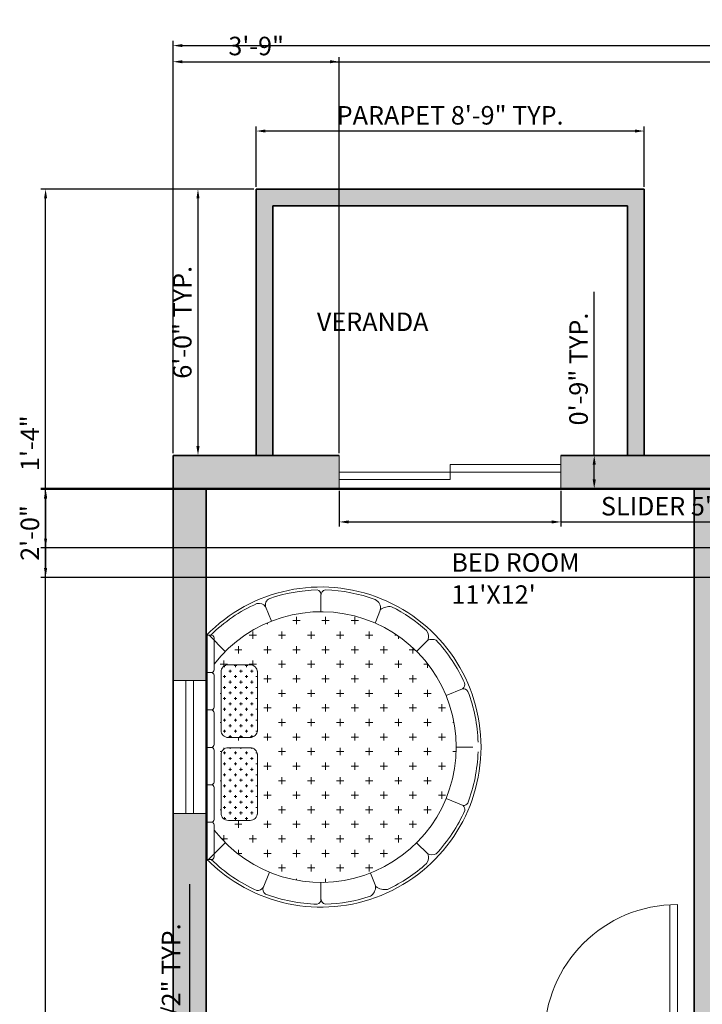
# Model space of a CAD drawing. Units: inches. Extents: x 2923 to 3500, y 1684 to 2381.
# Tile 10 of 12: x 2928 to 3112, y 2114 to 2380. Entities that reach past the tile are written whole.
import ezdxf

# ---------------------------------------------------------------- set-up
doc = ezdxf.new("R2010")
doc.units = ezdxf.units.IN
for name, color, linetype, lineweight in [('A-ANNO-DIMS', 2, 'Continuous', 18), ('A-AREA-IDEN', 7, 'Continuous', 18), ('A-DOOR', 3, 'Continuous', 18), ('A-FURN-PATT', 8, 'Continuous', 13), ('A-GLAZ', 4, 'Continuous', 18), ('A-WALL', 7, 'Continuous', 35), ('A-WALL-PATT', 9, 'Continuous', 13), ('Furniture', 7, 'Continuous', 15)]:
    doc.layers.add(name, color=color, linetype=linetype, lineweight=lineweight)
doc.styles.get("Standard").update_dxf_attribs({"font": 'txt', "height": 5})
doc.dimstyles.new('ISO-25', dxfattribs={"dimtxt": 5, "dimasz": 2.5, "dimexe": 1.25, "dimexo": 0.625, "dimtad": 1, "dimlunit": 3, "dimtxsty": 'Standard', "dimcen": 2.5, "dimadec": 0, "dimazin": 0, "dimtfac": 1, "dimtmove": 0, "dimatfit": 3, "dimfxl": 1, "dimarcsym": 0})

# ---------------------------------------------------------------- blocks, each defined once
blk = doc.blocks.new('*D2')
at = {"layer": 'A-ANNO-DIMS', "color": 0, "lineweight": -2, "transparency": 16777216}
for p, q in [((2969.23, 2263.03), (2969.23, 2374.52)), ((3397.23, 2263.03), (3397.23, 2374.52)), ((2971.73, 2373.27), (3394.73, 2373.27))]:
    blk.add_line(p, q, dxfattribs=at)
at = {"layer": 'A-ANNO-DIMS', "color": 0, "transparency": 16777216}
for points in [[(2971.73, 2373.69), (2971.73, 2372.86), (2969.23, 2373.27)], [(3394.73, 2373.69), (3394.73, 2372.86), (3397.23, 2373.27)]]:
    blk.add_solid(points, dxfattribs=at)
at = {"layer": 'Defpoints', "color": 0, "transparency": 16777216}
for p in [(3397.23, 2373.27), (2969.23, 2262.41), (3397.23, 2262.41)]:
    blk.add_point(p, dxfattribs=at)
at = {"layer": 'A-ANNO-DIMS', "color": 0, "transparency": 16777216, "insert": (3183.23, 2376.87), "char_height": 5, "attachment_point": 5}
blk.add_mtext('35\'-8"', dxfattribs=at)
blk = doc.blocks.new('DOOR-SINGLE-36IN')
for p, q in [((36, 36), (0, 36)), ((34, 0.06), (34, 36)), ((36, 0), (36, 36))]:
    blk.add_line(p, q)
blk.add_arc((36, 36), 36, 180, 270)
blk = doc.blocks.new('WINDOW-36IN')
for p, q in [((36, 9), (0, 9)), ((0, 9), (0, 0)), ((36, 0), (36, 9)), ((36, 5.5), (0, 5.5)), ((36, 3.5), (0, 3.5)), ((0, 0), (36, 0))]:
    blk.add_line(p, q)
blk = doc.blocks.new('WINDOW-SLIDING-60IN')
for p, q in [((0, 0), (0, 9)), ((60, 0), (60, 9)), ((30, 4.5), (30, 6.5)), ((30, 6.5), (60, 6.5)), ((60, 4.5), (0, 4.5)), ((30, 4.5), (30, 2.5)), ((30, 2.5), (0, 2.5))]:
    blk.add_line(p, q)
blk = doc.blocks.new('VERANDA-PARAPET')
for p, q in [((0, 72), (0, 0)), ((4.5, 72), (4.5, 4.5)), ((100.5, 72), (100.5, 4.5)), ((105, 72), (105, 0)), ((100.5, 4.5), (4.5, 4.5)), ((105, 0), (0, 0))]:
    blk.add_line(p, q)
blk = doc.blocks.new('BED-ROUND-FRAME')
for p, q in [((31.04, 79.92), (31.04, 84.58)), ((31.04, 79.92), (31.04, 84.58)), ((17.61, 77.37), (16.05, 81.29)), ((45.66, 76.84), (47.11, 80.49)), ((0, 13.11), (0, 73.51)), ((5.15, 69.2), (0.74, 73.61)), ((5.15, 69.2), (0.74, 73.61)), ((56.93, 69.2), (59.95, 72.21)), ((56.93, 69.2), (59.95, 72.21)), ((59.95, 72.21), (56.93, 69.2)), ((13.83, 63.84), (13.83, 47.62)), ((64.9, 57.24), (69.31, 59.05)), ((69.31, 59.05), (69.4, 59.09)), ((67.65, 43.31), (72.18, 43.31)), ((13.83, 41.4), (13.83, 25.18)), ((13.83, 39.13), (13.84, 39.12)), ((64.9, 29.37), (69.53, 27.47)), ((0.42, 12.68), (5.15, 17.42)), ((0.42, 12.68), (5.15, 17.42)), ((59.95, 14.4), (56.93, 17.42)), ((17.07, 9.46), (15.35, 5.25)), ((44.42, 9.23), (45.86, 5.58)), ((31.04, 1.98), (31.04, 6.69)), ((31.04, 2.04), (31.04, 6.69))]:
    blk.add_line(p, q)
for points in [[(4, 47.85), (4, 63.6, -0.414214), (5.97, 65.57), (11.88, 65.57, -0.414214), (13.84, 63.6), (13.84, 47.85, -0.414214), (11.88, 45.89), (5.97, 45.89, -0.414214)], [(4, 25.41), (4, 41.16, -0.414214), (5.97, 43.13), (11.88, 43.13, -0.414214), (13.84, 41.16), (13.84, 25.41, -0.414214), (11.88, 23.45), (5.97, 23.45, -0.414214)]]:
    blk.add_lwpolyline(points, format="xyb", close=True)
for centre, radius, start, end in [((31.04, 43.31), 43.31, 224.213, 135.787), ((31.04, 43.31), 42.52, 91.3819, 109.0292), ((29.76, 84.56), 1.29, 359.0498, 78.348), ((32.5, 84.36), 1.46, 98.688, 183.9778), ((31.04, 43.31), 42.52, 69.8397, 88.3303), ((17.88, 81.76), 1.88, 111.9527, 202.5488), ((44.67, 80.98), 2.46, 345.7709, 65.4979), ((31.04, 43.31), 42.52, 114.0695, 134.5949), ((31.04, 43.31), 36.61, 217.8198, 142.1802), ((14.23, 79.9), 2.29, 37.3562, 103.3498), ((49.64, 77.03), 4.29, 82.908, 126.1659), ((31.04, 43.31), 42.52, 47.802, 63.2705), ((57.53, 73.21), 2.61, 337.5919, 37.6583), ((61.1, 69.09), 3.33, 70.4217, 110.1689), ((31.04, 43.31), 42.52, 24.0703, 42.854), ((69.6, 57.73), 1.36, 26.1665, 102.6069), ((68.6, 60.18), 1.35, 304.4266, 20.4145), ((31.04, 43.31), 42.52, 1.7281, 20.7271), ((31.04, 43.31), 42.52, 339.0428, 358.2719), ((69.4, 29.21), 1.75, 274.2316, 320.4352), ((68.35, 26.36), 1.62, 353.6066, 43.1756), ((31.04, 43.31), 42.52, 317.146, 336.245), ((57.53, 13.4), 2.61, 322.3417, 22.4081), ((61.1, 17.52), 3.33, 249.8311, 289.5783), ((31.04, 43.31), 42.52, 225.7269, 245.8957), ((31.04, 43.31), 42.52, 295.113, 312.198), ((16.89, 4.85), 1.59, 153.9459, 235.5493), ((42.79, 5.51), 3.04, 302.4304, 3.4261), ((48.39, 9.04), 4.29, 233.8341, 279.2916), ((13.85, 6.32), 1.83, 264.4179, 326.0029), ((31.04, 43.31), 42.52, 249.2703, 268.6181), ((31.04, 43.31), 42.52, 271.6697, 288.3347), ((29.76, 2.06), 1.29, 281.652, 0.9502), ((32.5, 2.25), 1.46, 176.0222, 261.312)]:
    blk.add_arc(centre, radius, start, end)
blk = doc.blocks.new('*D21')
at = {"layer": 'A-ANNO-DIMS', "color": 0, "lineweight": -2, "transparency": 16777216}
for p, q in [((3014.23, 2252.78), (3014.23, 2243.16)), ((3074.23, 2252.78), (3074.23, 2243.16)), ((3016.73, 2244.41), (3071.73, 2244.41)), ((3074.23, 2244.41), (3148.22, 2244.41))]:
    blk.add_line(p, q, dxfattribs=at)
at = {"layer": 'A-ANNO-DIMS', "color": 0, "transparency": 16777216}
for points in [[(3016.73, 2244.82), (3016.73, 2243.99), (3014.23, 2244.41)], [(3071.73, 2244.82), (3071.73, 2243.99), (3074.23, 2244.41)]]:
    blk.add_solid(points, dxfattribs=at)
at = {"layer": 'Defpoints', "color": 0, "transparency": 16777216}
for p in [(3014.23, 2253.41), (3074.23, 2253.41), (3074.23, 2244.41)]:
    blk.add_point(p, dxfattribs=at)
at = {"layer": 'A-ANNO-DIMS', "color": 0, "transparency": 16777216, "insert": (3112.47, 2248.01), "char_height": 5, "attachment_point": 5}
blk.add_mtext('SLIDER 5\'-0" TYP.', dxfattribs=at)
blk = doc.blocks.new('*D22')
at = {"layer": 'A-ANNO-DIMS', "color": 0, "lineweight": -2, "transparency": 16777216}
for p, q in [((3083.23, 2262.41), (3083.23, 2306.63)), ((3074.85, 2262.41), (3084.48, 2262.41)), ((3083.23, 2255.91), (3083.23, 2259.91)), ((3074.85, 2253.41), (3084.48, 2253.41))]:
    blk.add_line(p, q, dxfattribs=at)
at = {"layer": 'A-ANNO-DIMS', "color": 0, "transparency": 16777216}
for points in [[(3082.81, 2259.91), (3083.65, 2259.91), (3083.23, 2262.41)], [(3082.81, 2255.91), (3083.65, 2255.91), (3083.23, 2253.41)]]:
    blk.add_solid(points, dxfattribs=at)
at = {"layer": 'Defpoints', "color": 0, "transparency": 16777216}
for p in [(3074.23, 2262.41), (3083.23, 2262.41), (3074.23, 2253.41)]:
    blk.add_point(p, dxfattribs=at)
at = {"layer": 'A-ANNO-DIMS', "color": 0, "transparency": 16777216, "insert": (3079.63, 2285.77), "char_height": 5, "attachment_point": 5, "rotation": 90}
blk.add_mtext('0\'-9" TYP.', dxfattribs=at)
blk = doc.blocks.new('*D31')
at = {"layer": 'A-ANNO-DIMS', "color": 0, "lineweight": -2, "transparency": 16777216}
for p, q in [((2991.73, 2335.03), (2991.73, 2351.41)), ((3094.23, 2350.16), (2994.23, 2350.16)), ((3096.73, 2335.03), (3096.73, 2351.41))]:
    blk.add_line(p, q, dxfattribs=at)
at = {"layer": 'A-ANNO-DIMS', "color": 0, "transparency": 16777216}
for points in [[(2994.23, 2350.57), (2994.23, 2349.74), (2991.73, 2350.16)], [(3094.23, 2350.57), (3094.23, 2349.74), (3096.73, 2350.16)]]:
    blk.add_solid(points, dxfattribs=at)
at = {"layer": 'Defpoints', "color": 0, "transparency": 16777216}
for p in [(2991.73, 2350.16), (2991.73, 2334.41), (3096.73, 2334.41)]:
    blk.add_point(p, dxfattribs=at)
at = {"layer": 'A-ANNO-DIMS', "color": 0, "transparency": 16777216, "insert": (3044.23, 2353.76), "char_height": 5, "attachment_point": 5}
blk.add_mtext('PARAPET 8\'-9" TYP.', dxfattribs=at)
blk = doc.blocks.new('*D32')
at = {"layer": 'A-ANNO-DIMS', "color": 0, "lineweight": -2, "transparency": 16777216}
for p, q in [((2991.1, 2334.41), (2974.73, 2334.41)), ((2975.98, 2331.91), (2975.98, 2264.91)), ((2991.1, 2262.41), (2974.73, 2262.41))]:
    blk.add_line(p, q, dxfattribs=at)
at = {"layer": 'A-ANNO-DIMS', "color": 0, "transparency": 16777216}
for points in [[(2975.56, 2331.91), (2976.4, 2331.91), (2975.98, 2334.41)], [(2975.56, 2264.91), (2976.4, 2264.91), (2975.98, 2262.41)]]:
    blk.add_solid(points, dxfattribs=at)
at = {"layer": 'Defpoints', "color": 0, "transparency": 16777216}
for p in [(2991.73, 2334.41), (2975.98, 2262.41), (2991.73, 2262.41)]:
    blk.add_point(p, dxfattribs=at)
at = {"layer": 'A-ANNO-DIMS', "color": 0, "transparency": 16777216, "insert": (2972.38, 2298.41), "char_height": 5, "attachment_point": 5, "rotation": 90}
blk.add_mtext('6\'-0" TYP.', dxfattribs=at)
blk = doc.blocks.new('*D35')
at = {"layer": 'A-ANNO-DIMS', "color": 0, "lineweight": -2, "transparency": 16777216}
for p, q in [((2973.77, 2068.57), (2973.77, 2146.37)), ((2977.6, 2068.57), (2972.52, 2068.57)), ((2973.77, 2041.37), (2973.77, 2066.07)), ((2977.6, 2038.87), (2972.52, 2038.87))]:
    blk.add_line(p, q, dxfattribs=at)
at = {"layer": 'A-ANNO-DIMS', "color": 0, "transparency": 16777216}
for points in [[(2973.36, 2066.07), (2974.19, 2066.07), (2973.77, 2068.57)], [(2973.36, 2041.37), (2974.19, 2041.37), (2973.77, 2038.87)]]:
    blk.add_solid(points, dxfattribs=at)
at = {"layer": 'Defpoints', "color": 0, "transparency": 16777216}
for p in [(2973.77, 2068.57), (2978.23, 2068.57), (2978.23, 2038.87)]:
    blk.add_point(p, dxfattribs=at)
at = {"layer": 'A-ANNO-DIMS', "color": 0, "transparency": 16777216, "insert": (2969.34, 2108.72), "char_height": 5, "attachment_point": 5, "rotation": 90}
blk.add_mtext('WC 2\'-5 1/2" TYP.', dxfattribs=at)
blk = doc.blocks.new('*D49')
at = {"layer": 'A-ANNO-DIMS', "color": 0, "lineweight": -2, "transparency": 16777216}
for p, q in [((2969.23, 2263.03), (2969.23, 2370.16)), ((2971.73, 2368.91), (3441.73, 2368.91)), ((3444.23, 2110.03), (3444.23, 2370.16))]:
    blk.add_line(p, q, dxfattribs=at)
at = {"layer": 'A-ANNO-DIMS', "color": 0, "transparency": 16777216}
for points in [[(2971.73, 2369.32), (2971.73, 2368.49), (2969.23, 2368.91)], [(3441.73, 2369.32), (3441.73, 2368.49), (3444.23, 2368.91)]]:
    blk.add_solid(points, dxfattribs=at)
at = {"layer": 'Defpoints', "color": 0, "transparency": 16777216}
for p in [(3444.23, 2368.91), (2969.23, 2262.41), (3444.23, 2109.41)]:
    blk.add_point(p, dxfattribs=at)
at = {"layer": 'A-ANNO-DIMS', "color": 0, "transparency": 16777216, "insert": (3206.73, 2372.51), "char_height": 5, "attachment_point": 5}
blk.add_mtext('39\'-7"', dxfattribs=at)
blk = doc.blocks.new('*D50')
at = {"layer": 'A-ANNO-DIMS', "color": 0, "lineweight": -2, "transparency": 16777216}
for p, q in [((2991.1, 2334.41), (2933.48, 2334.41)), ((2934.73, 1723.91), (2934.73, 2331.91)), ((3109.6, 1721.41), (2933.48, 1721.41))]:
    blk.add_line(p, q, dxfattribs=at)
at = {"layer": 'A-ANNO-DIMS', "color": 0, "transparency": 16777216}
for points in [[(2934.31, 2331.91), (2935.15, 2331.91), (2934.73, 2334.41)], [(2934.31, 1723.91), (2935.15, 1723.91), (2934.73, 1721.41)]]:
    blk.add_solid(points, dxfattribs=at)
at = {"layer": 'Defpoints', "color": 0, "transparency": 16777216}
for p in [(2934.73, 2334.41), (2991.73, 2334.41), (3110.23, 1721.41)]:
    blk.add_point(p, dxfattribs=at)
at = {"layer": 'A-ANNO-DIMS', "color": 0, "transparency": 16777216, "insert": (2931.13, 2027.91), "char_height": 5, "attachment_point": 5, "rotation": 90}
blk.add_mtext('51\'-1"', dxfattribs=at)
blk = doc.blocks.new('*D52')
at = {"layer": 'A-ANNO-DIMS', "color": 0, "lineweight": -2, "transparency": 16777216}
for p, q in [((3152.68, 2253.41), (2933.48, 2253.41)), ((2934.73, 2250.91), (2934.73, 2231.91)), ((3152.68, 2229.41), (2933.48, 2229.41))]:
    blk.add_line(p, q, dxfattribs=at)
at = {"layer": 'A-ANNO-DIMS', "color": 0, "transparency": 16777216}
for points in [[(2934.31, 2250.91), (2935.15, 2250.91), (2934.73, 2253.41)], [(2934.31, 2231.91), (2935.15, 2231.91), (2934.73, 2229.41)]]:
    blk.add_solid(points, dxfattribs=at)
at = {"layer": 'Defpoints', "color": 0, "transparency": 16777216}
for p in [(3153.3, 2253.41), (2934.73, 2229.41), (3153.3, 2229.41)]:
    blk.add_point(p, dxfattribs=at)
at = {"layer": 'A-ANNO-DIMS', "color": 0, "transparency": 16777216, "insert": (2931.13, 2241.41), "char_height": 5, "attachment_point": 5, "rotation": 90}
blk.add_mtext('2\'-0"', dxfattribs=at)
blk = doc.blocks.new('*D55')
at = {"layer": 'A-ANNO-DIMS', "color": 0, "lineweight": -2, "transparency": 16777216}
for p, q in [((2934.73, 2253.17), (2934.73, 2275.73)), ((3165.61, 2253.17), (2933.48, 2253.17)), ((2934.73, 2239.88), (2934.73, 2250.67)), ((3165.69, 2237.38), (2933.48, 2237.38))]:
    blk.add_line(p, q, dxfattribs=at)
at = {"layer": 'A-ANNO-DIMS', "color": 0, "transparency": 16777216}
for points in [[(2934.31, 2250.67), (2935.15, 2250.67), (2934.73, 2253.17)], [(2934.31, 2239.88), (2935.15, 2239.88), (2934.73, 2237.38)]]:
    blk.add_solid(points, dxfattribs=at)
at = {"layer": 'Defpoints', "color": 0, "transparency": 16777216}
for p in [(2934.73, 2253.17), (3166.23, 2253.17), (3166.32, 2237.38)]:
    blk.add_point(p, dxfattribs=at)
at = {"layer": 'A-ANNO-DIMS', "color": 0, "transparency": 16777216, "insert": (2931.13, 2265.7), "char_height": 5, "attachment_point": 5, "rotation": 90}
blk.add_mtext('1\'-4"', dxfattribs=at)
blk = doc.blocks.new('*D58')
at = {"layer": 'A-ANNO-DIMS', "color": 0, "lineweight": -2, "transparency": 16777216}
for p, q in [((2969.23, 2263.03), (2969.23, 2370.16)), ((2971.73, 2368.91), (3011.73, 2368.91)), ((3014.23, 2263.03), (3014.23, 2370.16))]:
    blk.add_line(p, q, dxfattribs=at)
at = {"layer": 'A-ANNO-DIMS', "color": 0, "transparency": 16777216}
for points in [[(2971.73, 2369.32), (2971.73, 2368.49), (2969.23, 2368.91)], [(3011.73, 2369.32), (3011.73, 2368.49), (3014.23, 2368.91)]]:
    blk.add_solid(points, dxfattribs=at)
at = {"layer": 'Defpoints', "color": 0, "transparency": 16777216}
for p in [(3014.23, 2368.91), (2969.23, 2262.41), (3014.23, 2262.41)]:
    blk.add_point(p, dxfattribs=at)
at = {"layer": 'A-ANNO-DIMS', "color": 0, "transparency": 16777216, "insert": (2991.73, 2372.51), "char_height": 5, "attachment_point": 5}
blk.add_mtext('3\'-9"', dxfattribs=at)

msp = doc.modelspace()

# ---------------------------------------------------------------- hatches: boundary and pattern name
at = {"layer": 'A-FURN-PATT'}
h = msp.add_hatch(dxfattribs=at)
h.set_pattern_fill('CROSS', color=256, scale=15.748, angle=180, style=0)
h.set_pattern_definition([(360, (1245.7636, 674.407), (3.937, -3.937), [1.9685, -5.9055]), (270, (1246.748, 675.3913), (-3.937, -3.937), [1.9685, -5.9055])])
h.paths.add_polyline_path([(2980.347, 2205.951), (2980.347, 2203.657), (2979.599, 2203.657, -0.4142136), (2980.347, 2202.909), (2980.347, 2193.537), (2979.599, 2193.537, -0.4142136), (2980.347, 2192.789), (2980.347, 2183.417), (2979.599, 2183.417, -0.4142136), (2980.347, 2182.669), (2980.347, 2173.296), (2979.599, 2173.296, -0.4142136), (2980.347, 2172.548), (2980.347, 2163.176), (2979.599, 2163.176, -0.4142136), (2980.347, 2162.428), (2980.347, 2161.049, 2.9191153)])
h.paths.add_polyline_path([(2992.074, 2165.606, -0.4142136), (2990.105, 2163.638), (2984.2, 2163.638, -0.4142136), (2982.231, 2165.606), (2982.231, 2181.354, -0.4142136), (2984.2, 2183.323), (2990.105, 2183.323, -0.4142136), (2992.074, 2181.354)], flags=16)
h.paths.add_polyline_path([(2992.074, 2188.047, -0.4142136), (2990.105, 2186.079), (2984.2, 2186.079, -0.4142136), (2982.231, 2188.047), (2982.231, 2203.795, -0.4142136), (2984.2, 2205.764), (2990.105, 2205.764, -0.4142136), (2992.074, 2203.795)], flags=16)
h = msp.add_hatch(dxfattribs=at)
h.set_pattern_fill('CROSS', color=256, scale=5.9055, angle=450, style=0)
h.set_pattern_definition([(90, (3722.8477, 1506.83), (-1.476375, 1.476375), [0.7381875, -2.2145625]), (180, (3723.2168, 1507.1991), (-1.476375, -1.476375), [0.7381875, -2.2145625])])
h.paths.add_polyline_path([(2982.231, 2165.606, 0.4142136), (2984.2, 2163.638), (2990.105, 2163.638, 0.4142136), (2992.074, 2165.606), (2992.074, 2181.354, 0.4142136), (2990.105, 2183.323), (2984.2, 2183.323, 0.4142136), (2982.231, 2181.354)])
h.paths.add_polyline_path([(2992.074, 2203.795, 0.4142136), (2990.105, 2205.764), (2984.2, 2205.764, 0.4142136), (2982.231, 2203.795), (2982.231, 2188.047, 0.4142136), (2984.2, 2186.079), (2990.105, 2186.079, 0.4142136), (2992.074, 2188.047)])
at = {"layer": 'A-WALL-PATT'}
h = msp.add_hatch(color=256, dxfattribs=at)
h.dxf.hatch_style = 1
h.paths.add_polyline_path([(3014.23, 2262.406), (2969.23, 2262.406), (2969.23, 2201.5), (2978.23, 2201.5), (2978.23, 2213.699), (2978.23, 2253.406), (3014.23, 2253.406)])
h.paths.add_polyline_path([(3119.23, 2262.406), (3074.23, 2262.406), (3074.23, 2253.406), (3110.23, 2253.406), (3110.23, 2109.406), (3105.73, 2109.406), (3105.73, 2104.906), (3114.73, 2104.906), (3114.73, 2152.906), (3119.23, 2152.906), (3119.23, 2157.406), (3114.73, 2157.406), (3114.73, 2253.406), (3119.23, 2253.406)])
h.paths.add_polyline_path([(3179.98, 2262.406), (3149.23, 2262.406), (3149.23, 2253.406), (3179.98, 2253.406)], flags=0)
h.paths.add_polyline_path([(3295.73, 2262.406), (3215.98, 2262.406), (3215.98, 2253.406), (3246.73, 2253.406), (3246.73, 2157.406), (3149.23, 2157.406), (3149.23, 2152.906), (3246.73, 2152.906), (3246.73, 2149.906), (3251.23, 2149.906), (3251.23, 2253.406), (3295.73, 2253.406)])
h.paths.add_polyline_path([(3397.23, 2262.406), (3343.73, 2262.406), (3343.73, 2253.406), (3349.929, 2253.406), (3388.23, 2253.406), (3388.23, 2199.406), (3397.23, 2199.406)])
h.paths.add_polyline_path([(3369.935, 2334.406), (3264.935, 2334.406), (3264.935, 2262.406), (3269.435, 2262.406), (3269.435, 2329.906), (3365.435, 2329.906), (3365.435, 2262.406), (3369.935, 2262.406)])
h.paths.add_polyline_path([(3096.73, 2334.406), (2991.73, 2334.406), (2991.73, 2262.406), (2996.23, 2262.406), (2996.23, 2329.906), (3092.23, 2329.906), (3092.23, 2262.406), (3096.73, 2262.406)])
h.paths.add_polyline_path([(3397.23, 2163.406), (3388.23, 2163.406), (3388.23, 2109.406), (3251.23, 2109.406), (3251.23, 2113.906), (3246.73, 2113.906), (3246.73, 2092.906), (3251.23, 2092.906), (3251.23, 2104.906), (3435.23, 2104.906), (3435.23, 2080.906), (3444.23, 2080.906), (3444.23, 2109.406), (3397.23, 2109.406)])
h.paths.add_polyline_path([(3444.23, 2044.906), (3435.23, 2044.906), (3435.23, 2020.906), (3251.23, 2020.906), (3251.23, 2032.906), (3246.73, 2032.906), (3246.73, 2016.406), (3251.23, 2016.406), (3287.73, 2016.406), (3287.73, 1968.406), (3287.23, 1968.406), (3287.23, 1963.906), (3296.73, 1963.906), (3296.73, 1968.406), (3292.23, 1968.406), (3292.23, 2016.406), (3388.23, 2016.406), (3388.23, 2004.398), (3397.23, 2004.398), (3397.23, 2016.406), (3444.23, 2016.406)])
h.paths.add_polyline_path([(3397.23, 1980.398), (3388.23, 1980.398), (3388.23, 1979.998), (3388.23, 1969.828), (3388.23, 1968.406), (3326.73, 1968.406), (3326.73, 1963.906), (3388.23, 1963.906), (3388.23, 1913.156), (3397.23, 1913.156)])
h.paths.add_polyline_path([(3251.23, 1968.406), (3150.73, 1968.406), (3150.73, 1963.906), (3246.73, 1963.906), (3246.73, 1826.406), (3230.98, 1826.406), (3230.98, 1817.406), (3251.23, 1817.406), (3251.23, 1963.906)])
h.paths.add_polyline_path([(3114.73, 1968.406), (3105.73, 1968.406), (3105.73, 1963.906), (3110.23, 1963.906), (3110.23, 1817.406), (3119.23, 1817.406), (3119.23, 1826.406), (3114.73, 1826.406)])
h.paths.add_polyline_path([(3069.73, 1968.406), (3066.73, 1968.406), (3066.73, 1972.906), (3062.23, 1972.906), (3062.23, 1968.406), (2978.23, 1968.406), (2978.23, 1989.406), (2969.23, 1989.406), (2969.23, 1912.505), (2978.23, 1912.505), (2978.23, 1925.355), (2978.23, 1963.906), (3069.73, 1963.906)])
h.paths.add_polyline_path([(3066.73, 2104.906), (3069.73, 2104.906), (3069.73, 2109.406), (3057.73, 2109.406), (3057.73, 2104.906), (3062.23, 2104.906), (3062.23, 2038.906), (2978.23, 2038.906), (2978.23, 2059.906), (2969.23, 2059.906), (2969.23, 2013.406), (2978.23, 2013.406), (2978.23, 2034.406), (3062.23, 2034.406), (3062.23, 2002.906), (3066.73, 2002.906)])
h.paths.add_polyline_path([(3027.73, 2109.406), (2978.23, 2109.406), (2978.23, 2165.5), (2969.23, 2165.5), (2969.23, 2083.906), (2978.23, 2083.906), (2978.23, 2104.906), (3027.73, 2104.906)])
h.paths.add_polyline_path([(2978.23, 1876.505), (2969.23, 1876.505), (2969.23, 1817.406), (3014.23, 1817.406), (3014.23, 1826.406), (2978.23, 1826.406)])
h.paths.add_polyline_path([(2996.23, 1817.406), (2991.73, 1817.406), (2991.73, 1745.406), (3096.73, 1745.406), (3096.73, 1817.406), (3092.23, 1817.406), (3092.23, 1749.906), (2996.23, 1749.906)])
h.paths.add_polyline_path([(3289.73, 1826.406), (3251.23, 1826.406), (3251.23, 1817.406), (3289.73, 1817.406)])
h.paths.add_polyline_path([(3397.23, 1877.156), (3388.23, 1877.156), (3388.23, 1864.957), (3388.23, 1826.406), (3349.73, 1826.406), (3349.73, 1817.406), (3397.23, 1817.406)])
h.paths.add_polyline_path([(3374.267, 1817.406), (3369.767, 1817.406), (3369.767, 1749.906), (3273.767, 1749.906), (3273.767, 1817.406), (3269.267, 1817.406), (3269.267, 1745.406), (3374.267, 1745.406)])

# ---------------------------------------------------------------- linework, layer by layer
at = {"layer": 'A-WALL'}
for p, q in [((2969.23, 2262.406), (3014.23, 2262.406)), ((2969.23, 1817.406), (2969.23, 2262.406)), ((3074.23, 2262.406), (3119.23, 2262.406)), ((2978.23, 2253.406), (3014.23, 2253.406)), ((2978.23, 2109.406), (2978.23, 2253.406)), ((3074.23, 2253.406), (3110.23, 2253.406)), ((3110.23, 2109.406), (3110.23, 2253.406))]:
    msp.add_line(p, q, dxfattribs=at)
at = {"layer": 'Furniture'}
for points in [[(2980.347, 2204.405), (2980.347, 2213.03, 0.4142136), (2979.599, 2213.778), (2978.458, 2213.778), (2978.458, 2203.657), (2979.599, 2203.657, 0.4142136)], [(2980.347, 2194.285), (2980.347, 2202.909, 0.4142136), (2979.599, 2203.657), (2978.458, 2203.657), (2978.458, 2193.537), (2979.599, 2193.537, 0.4142136)], [(2980.347, 2184.165), (2980.347, 2192.789, 0.4142136), (2979.599, 2193.537), (2978.458, 2193.537), (2978.458, 2183.417), (2979.599, 2183.417, 0.4142136)], [(2980.347, 2174.044), (2980.347, 2182.669, 0.4142136), (2979.599, 2183.417), (2978.458, 2183.417), (2978.458, 2173.296), (2979.599, 2173.296, 0.4142136)], [(2980.347, 2163.924), (2980.347, 2172.548, 0.4142136), (2979.599, 2173.296), (2978.458, 2173.296), (2978.458, 2163.176), (2979.599, 2163.176, 0.4142136)], [(2980.347, 2153.803), (2980.347, 2162.428, 0.4142136), (2979.599, 2163.176), (2978.458, 2163.176), (2978.458, 2153.055), (2979.599, 2153.055, 0.4142136)]]:
    msp.add_lwpolyline(points, format="xyb", close=True, dxfattribs=at)

# ---------------------------------------------------------------- block references
at = {"layer": 'A-DOOR', "extrusion": (0, 0, -1), "zscale": -1, "rotation": 180}
msp.add_blockref('DOOR-SINGLE-36IN', (-3069.73, 2140.906), dxfattribs=at)
at = {"layer": 'A-GLAZ'}
msp.add_blockref('WINDOW-SLIDING-60IN', (3014.23, 2253.406), dxfattribs=at)
at = {"layer": 'A-GLAZ', "rotation": 269.9999999999969}
msp.add_blockref('WINDOW-36IN', (2969.23, 2201.5), dxfattribs=at)
at = {"layer": 'A-WALL', "rotation": 180}
msp.add_blockref('VERANDA-PARAPET', (3096.73, 2334.406), dxfattribs=at)
at = {"layer": 'Furniture'}
msp.add_blockref('BED-ROUND-FRAME', (2978.23, 2140.193), dxfattribs=at)

# ---------------------------------------------------------------- texts
at = {"layer": 'A-AREA-IDEN'}
for s, p in [('VERANDA', (3008.163, 2296.062)), ('BED ROOM', (3044.544, 2230.948)), ("11'X12'", (3044.544, 2222.263))]:
    msp.add_text(s, height=5, dxfattribs=at).set_placement(p)

# ---------------------------------------------------------------- dimensions: what is measured, and where the dimension line sits
at = {"layer": 'A-ANNO-DIMS'}
for base, p2, override, picture, middle in [((3397.23, 2373.272), (3397.23, 2262.406), {"dimclrd": 0, "dimclre": 0, "dimclrt": 0}, '*D2', (3183.23, 2376.874)), ((3444.23, 2368.906), (3444.23, 2109.406), {"dimdec": 1, "dimlfac": 1, "dimrnd": 0, "dimzin": 1, "dimdsep": 46, "dimlunit": 4, "dimfrac": 2}, '*D49', (3206.73, 2372.507)), ((3014.23, 2368.906), (3014.23, 2262.406), {"dimdec": 1, "dimlfac": 1, "dimrnd": 0, "dimzin": 1, "dimdsep": 46, "dimlunit": 4, "dimfrac": 2}, '*D58', (2991.73, 2372.507))]:
    dim = msp.add_linear_dim(base=base, p1=(2969.23, 2262.406), p2=p2, dimstyle='ISO-25', override=override, dxfattribs=at)
    dim.commit()
    dim.dimension.update_dxf_attribs({"geometry": picture, "text_midpoint": middle})
for base, p1, p2, angle, text, picture, middle in [((2991.73, 2350.156), (3096.73, 2334.406), (2991.73, 2334.406), 180, 'PARAPET <> TYP.', '*D31', (3044.23, 2353.757)), ((2975.98, 2262.406), (2991.73, 2334.406), (2991.73, 2262.406), 270, '<> TYP.', '*D32', (2972.379, 2298.406)), ((3083.23, 2262.406), (3074.23, 2253.406), (3074.23, 2262.406), 90, '<> TYP.', '*D22', (3079.629, 2285.769)), ((2973.775, 2068.571), (2978.23, 2038.87), (2978.23, 2068.571), 90, 'WC <> TYP.', '*D35', (2969.34, 2108.72))]:
    dim = msp.add_linear_dim(base=base, p1=p1, p2=p2, angle=angle, text=text, dimstyle='ISO-25', override={"dimdec": 1, "dimlfac": 1, "dimrnd": 0, "dimzin": 1, "dimdsep": 46, "dimlunit": 4, "dimfrac": 2}, dxfattribs=at)
    dim.commit()
    dim.dimension.update_dxf_attribs({"geometry": picture, "text_midpoint": middle})
for base, p1, p2, picture, middle in [((2934.73, 2334.406), (3110.23, 1721.406), (2991.73, 2334.406), '*D50', (2931.129, 2027.906)), ((2934.73, 2253.166), (3166.316, 2237.38), (3166.231, 2253.166), '*D55', (2931.129, 2265.696)), ((2934.73, 2229.406), (3153.303, 2253.406), (3153.303, 2229.406), '*D52', (2931.129, 2241.406))]:
    dim = msp.add_linear_dim(base=base, p1=p1, p2=p2, angle=90, dimstyle='ISO-25', override={"dimdec": 1, "dimlfac": 1, "dimrnd": 0, "dimzin": 1, "dimdsep": 46, "dimlunit": 4, "dimfrac": 2}, dxfattribs=at)
    dim.commit()
    dim.dimension.update_dxf_attribs({"geometry": picture, "text_midpoint": middle})
dim = msp.add_linear_dim(base=(3074.23, 2244.406), p1=(3014.23, 2253.406), p2=(3074.23, 2253.406), text='SLIDER <> TYP.', dimstyle='ISO-25', override={"dimdec": 1, "dimlfac": 1, "dimrnd": 0, "dimzin": 1, "dimdsep": 46, "dimlunit": 4, "dimfrac": 2}, dxfattribs=at)
dim.commit()
dim.dimension.update_dxf_attribs({"geometry": '*D21', "text_midpoint": (3112.474, 2248.007)})

doc.saveas('drawing.dxf')
